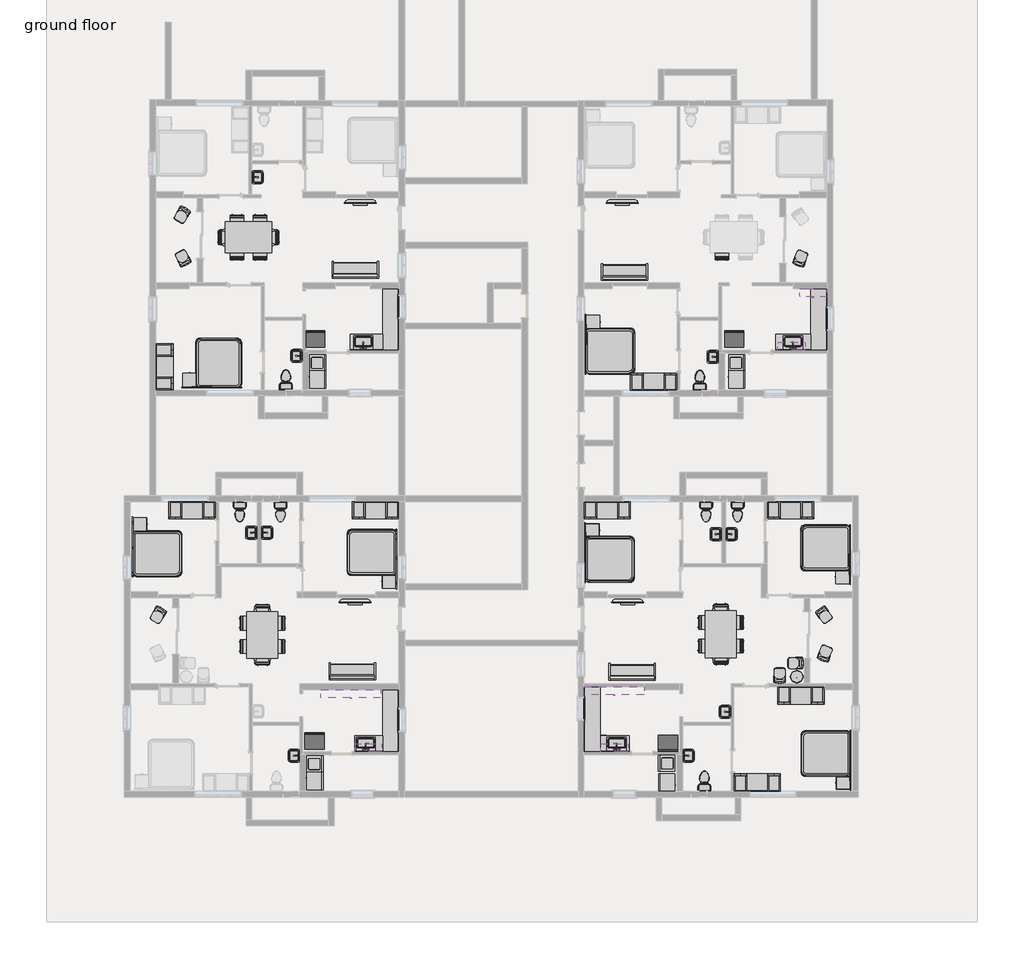
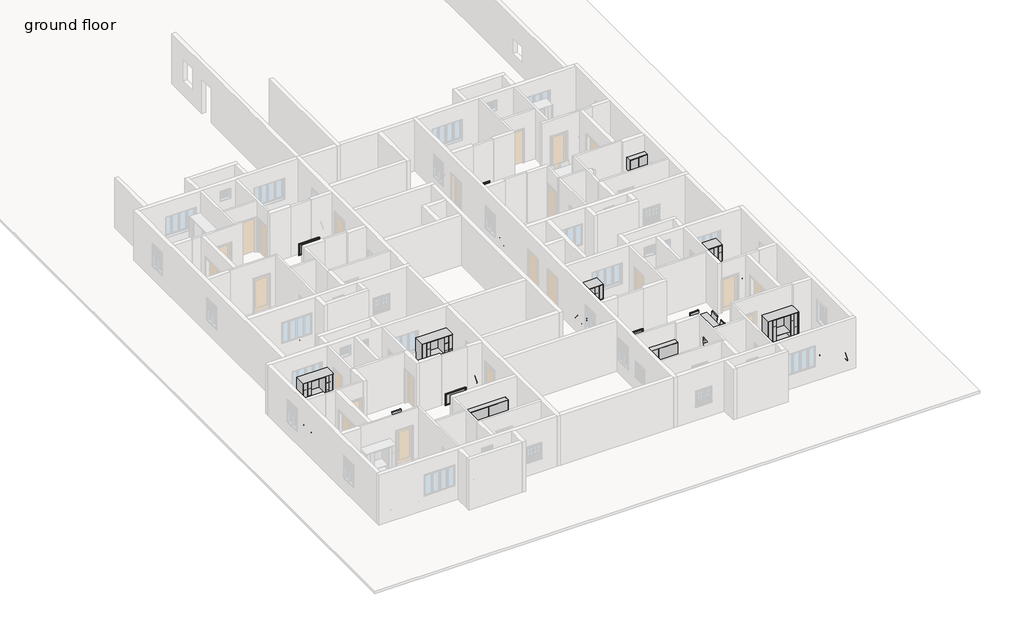
# One storey, part 11 of 16: 80 furniture elements, 21 flow terminals, 12 proxies.
"""IFC4 building model written with IfcOpenShell, lengths in millimetres."""

from ifc_helpers import new_model, si_unit, origin, place, context, project, spatial, transform, mapped, element, save
from components import proxy_97c73763, proxy_19935bb1, proxy_76352e5b, proxy_1934c8a4, flow_terminal_4d548711, flow_terminal_8d9ea526, toilet_domestic_3d_toilet_domestic_3d_ba6479b0, toilet_domestic_3d_toilet_domestic_3d_30431060, bed_design_8999_bed_design_8999_9c973422, bed_design_8999_bed_design_8999_e911dec7, furniture_f87f75a4, furniture_a56de0b1, furniture_97fe820d, furniture_007fecef, chair_task_chair_task_b7f3823b, chair_task_arms_chair_task_arms_fa5a08ef, furniture_bc399e91, furniture_0b9e3d50, furniture_ce4e80af, furniture_8ade2860, furniture_1cc325eb, furniture_015143fb, furniture_88072bd9, furniture_eb3a3c23, furniture_4fdbbe14, furniture_57f9710a, furniture_0b81fedb, furniture_0bcc43ae, furniture_3dd5e188, furniture_9929ec1f, furniture_f73e1c42, furniture_a4bc473d, furniture_3df5d44a

model = new_model("IFC4")

# Units and contexts
model_context = context("Model", 3, world=origin())
ifc_project = project(units=[si_unit("LENGTHUNIT", "METRE", prefix="MILLI")], contexts=[model_context])

# Site, building, storey
site = spatial("IfcSite", under=ifc_project)
building = spatial("IfcBuilding", under=site)
storey = spatial("IfcBuildingStorey", under=building, Name="ground floor", Elevation=609.6)

# Proxies
placement = place(None, origin())
proxy_shape = proxy_97c73763(model_context)
element("IfcBuildingElementProxy", 1, Name="Dryer : 27\" x 25\" x 35\"", ObjectType="Dryer : 27\" x 25\" x 35\"", at=placement, inside=storey, context=model_context, shape_type="MappedRepresentation", body=[
    mapped(proxy_shape, transform((48815.0055897, -8570.7128329, 609.6), x_axis=(0.0, -1.0, 0.0), y_axis=(1.0, 0.0, 0.0), z_axis=(0.0, 0.0, 1.0))),
])
element("IfcBuildingElementProxy", 2, Name="Dryer : 27\" x 25\" x 35\"", ObjectType="Dryer : 27\" x 25\" x 35\"", at=placement, inside=storey, context=model_context, shape_type="MappedRepresentation", body=[
    mapped(proxy_shape, transform((65274.2055897, -8570.7128329, 609.6), x_axis=(0.0, -1.0, 0.0), y_axis=(1.0, 0.0, 0.0), z_axis=(0.0, 0.0, 1.0))),
])
element("IfcBuildingElementProxy", 3, Name="Dryer : 27\" x 25\" x 35\"", ObjectType="Dryer : 27\" x 25\" x 35\"", at=placement, inside=storey, context=model_context, shape_type="MappedRepresentation", body=[
    mapped(proxy_shape, transform((63151.1859463, -25146.6240794, 609.6), x_axis=(0.0, 1.0, 0.0), y_axis=(-1.0, 0.0, 0.0), z_axis=(0.0, 0.0, 1.0))),
])
element("IfcBuildingElementProxy", 4, Name="Dryer : 27\" x 25\" x 35\"", ObjectType="Dryer : 27\" x 25\" x 35\"", at=placement, inside=storey, context=model_context, shape_type="MappedRepresentation", body=[
    mapped(proxy_shape, transform((48702.4341432, -24333.8240794, 609.6), x_axis=(0.0, -1.0, 0.0), y_axis=(1.0, 0.0, 0.0), z_axis=(0.0, 0.0, 1.0))),
])
proxy_2_shape = proxy_19935bb1(model_context)
element("IfcBuildingElementProxy", 5, Name="Refrigerator-Built-in : 30\" x 24\" LH", ObjectType="Refrigerator-Built-in : 30\" x 24\" LH", at=placement, inside=storey, context=model_context, shape_type="MappedRepresentation", body=[
    mapped(proxy_2_shape, transform((62887.9133315, -23204.1520196, 609.6), x_axis=(1.0, 0.0, 0.0), y_axis=(0.0, 1.0, 0.0), z_axis=(0.0, 0.0, 1.0))),
])
proxy_3_shape = proxy_76352e5b(model_context)
element("IfcBuildingElementProxy", 6, Name="Refrigerator-Built-in : 30\" x 24\" LH", ObjectType="Refrigerator-Built-in : 30\" x 24\" LH", at=placement, inside=storey, context=model_context, shape_type="MappedRepresentation", body=[
    mapped(proxy_3_shape, transform((49034.332975, -7390.2407731, 609.6), x_axis=(1.0, 0.0, 0.0), y_axis=(0.0, 1.0, 0.0), z_axis=(0.0, 0.0, 1.0))),
])
element("IfcBuildingElementProxy", 7, Name="Refrigerator-Built-in : 30\" x 24\" LH", ObjectType="Refrigerator-Built-in : 30\" x 24\" LH", at=placement, inside=storey, context=model_context, shape_type="MappedRepresentation", body=[
    mapped(proxy_3_shape, transform((65493.532975, -7390.2407731, 609.6), x_axis=(1.0, 0.0, 0.0), y_axis=(0.0, 1.0, 0.0), z_axis=(0.0, 0.0, 1.0))),
])
element("IfcBuildingElementProxy", 8, Name="Refrigerator-Built-in : 30\" x 24\" LH", ObjectType="Refrigerator-Built-in : 30\" x 24\" LH", at=placement, inside=storey, context=model_context, shape_type="MappedRepresentation", body=[
    mapped(proxy_3_shape, transform((48997.9615284, -23178.7520196, 609.6), x_axis=(1.0, 0.0, 0.0), y_axis=(0.0, 1.0, 0.0), z_axis=(0.0, 0.0, 1.0))),
])
proxy_4_shape = proxy_1934c8a4(model_context)
element("IfcBuildingElementProxy", 9, Name="Washer : 25\" x 25\" x 35\"", ObjectType="Washer : 25\" x 25\" x 35\"", at=placement, inside=storey, context=model_context, shape_type="MappedRepresentation", body=[
    mapped(proxy_4_shape, transform((48850.5170287, -7894.2828207, 609.6), x_axis=(0.0, -1.0, 0.0), y_axis=(1.0, 0.0, 0.0), z_axis=(0.0, 0.0, 1.0))),
])
element("IfcBuildingElementProxy", 10, Name="Washer : 25\" x 25\" x 35\"", ObjectType="Washer : 25\" x 25\" x 35\"", at=placement, inside=storey, context=model_context, shape_type="MappedRepresentation", body=[
    mapped(proxy_4_shape, transform((65309.7170287, -7894.2828207, 609.6), x_axis=(0.0, -1.0, 0.0), y_axis=(1.0, 0.0, 0.0), z_axis=(0.0, 0.0, 1.0))),
])
element("IfcBuildingElementProxy", 11, Name="Washer : 25\" x 25\" x 35\"", ObjectType="Washer : 25\" x 25\" x 35\"", at=placement, inside=storey, context=model_context, shape_type="MappedRepresentation", body=[
    mapped(proxy_4_shape, transform((63110.4973853, -24419.3940673, 609.6), x_axis=(0.0, 1.0, 0.0), y_axis=(-1.0, 0.0, 0.0), z_axis=(0.0, 0.0, 1.0))),
])
element("IfcBuildingElementProxy", 12, Name="Washer : 25\" x 25\" x 35\"", ObjectType="Washer : 25\" x 25\" x 35\"", at=placement, inside=storey, context=model_context, shape_type="MappedRepresentation", body=[
    mapped(proxy_4_shape, transform((48737.9455822, -23657.3940673, 609.6), x_axis=(0.0, -1.0, 0.0), y_axis=(1.0, 0.0, 0.0), z_axis=(0.0, 0.0, 1.0))),
])

# Flow terminals
flow_terminal_shape = flow_terminal_4d548711(model_context)
element("IfcFlowTerminal", 13, ObjectType="Sink Kitchen-Single : 30\" x 21\"", at=placement, inside=storey, context=model_context, shape_type="MappedRepresentation", body=[
    mapped(flow_terminal_shape, transform((50929.549914, -7494.5659653, 609.6), x_axis=(-1.0, 0.0, 0.0), y_axis=(0.0, -1.0, 0.0), z_axis=(0.0, 0.0, 1.0))),
])
element("IfcFlowTerminal", 14, ObjectType="Sink Kitchen-Single : 30\" x 21\"", at=placement, inside=storey, context=model_context, shape_type="MappedRepresentation", body=[
    mapped(flow_terminal_shape, transform((67814.4575644, -7494.5659653, 609.6), x_axis=(-1.0, 0.0, 0.0), y_axis=(0.0, -1.0, 0.0), z_axis=(0.0, 0.0, 1.0))),
])
element("IfcFlowTerminal", 15, ObjectType="Sink Kitchen-Single : 30\" x 21\"", at=placement, inside=storey, context=model_context, shape_type="MappedRepresentation", body=[
    mapped(flow_terminal_shape, transform((60886.6970546, -23264.1704575, 609.6), x_axis=(-1.0, 0.0, 0.0), y_axis=(0.0, -1.0, 0.0), z_axis=(0.0, 0.0, 1.0))),
])
element("IfcFlowTerminal", 16, ObjectType="Sink Kitchen-Single : 30\" x 21\"", at=placement, inside=storey, context=model_context, shape_type="MappedRepresentation", body=[
    mapped(flow_terminal_shape, transform((51027.9054731, -23264.2911897, 609.6), x_axis=(-1.0, 0.0, 0.0), y_axis=(0.0, -1.0, 0.0), z_axis=(0.0, 0.0, 1.0))),
])
flow_terminal_2_shape = flow_terminal_8d9ea526(model_context)
element("IfcFlowTerminal", 17, ObjectType="Sink Vanity-Square : 20\" x 18\"", at=placement, inside=storey, context=model_context, shape_type="MappedRepresentation", body=[
    mapped(flow_terminal_2_shape, transform((64700.8858807, -8040.0221259, 609.6), x_axis=(0.0, -1.0, 0.0), y_axis=(1.0, 0.0, 0.0), z_axis=(0.0, 0.0, 1.0))),
])
element("IfcFlowTerminal", 18, ObjectType="Sink Vanity-Square : 20\" x 18\"", at=placement, inside=storey, context=model_context, shape_type="MappedRepresentation", body=[
    mapped(flow_terminal_2_shape, transform((64819.063292, -15003.2055572, 609.6), x_axis=(0.0, -1.0, 0.0), y_axis=(1.0, 0.0, 0.0), z_axis=(0.0, 0.0, 1.0))),
])
element("IfcFlowTerminal", 19, ObjectType="Sink Vanity-Square : 20\" x 18\"", at=placement, inside=storey, context=model_context, shape_type="MappedRepresentation", body=[
    mapped(flow_terminal_2_shape, transform((65325.5370757, -15034.5840384, 609.6), x_axis=(0.0, 1.0, 0.0), y_axis=(-1.0, 0.0, 0.0), z_axis=(0.0, 0.0, 1.0))),
])
element("IfcFlowTerminal", 20, ObjectType="Sink Vanity-Square : 20\" x 18\"", at=placement, inside=storey, context=model_context, shape_type="MappedRepresentation", body=[
    mapped(flow_terminal_2_shape, transform((65180.5928441, -21983.9881535, 609.6), x_axis=(0.0, -1.0, 0.0), y_axis=(1.0, 0.0, 0.0), z_axis=(0.0, 0.0, 1.0))),
])
element("IfcFlowTerminal", 21, ObjectType="Sink Vanity-Square : 20\" x 18\"", at=placement, inside=storey, context=model_context, shape_type="MappedRepresentation", body=[
    mapped(flow_terminal_2_shape, transform((63638.776683, -23739.4050992, 609.6), x_axis=(0.0, 1.0, 0.0), y_axis=(-1.0, 0.0, 0.0), z_axis=(0.0, 0.0, 1.0))),
])
element("IfcFlowTerminal", 22, ObjectType="Sink Vanity-Square : 20\" x 18\"", at=placement, inside=storey, context=model_context, shape_type="MappedRepresentation", body=[
    mapped(flow_terminal_2_shape, transform((48244.6808419, -23708.1473503, 609.6), x_axis=(0.0, -1.0, 0.0), y_axis=(1.0, 0.0, 0.0), z_axis=(0.0, 0.0, 1.0))),
])
element("IfcFlowTerminal", 23, ObjectType="Sink Vanity-Square : 20\" x 18\"", at=placement, inside=storey, context=model_context, shape_type="MappedRepresentation", body=[
    mapped(flow_terminal_2_shape, transform((46567.622986, -14945.2984998, 609.6), x_axis=(0.0, -1.0, 0.0), y_axis=(1.0, 0.0, 0.0), z_axis=(0.0, 0.0, 1.0))),
])
element("IfcFlowTerminal", 24, ObjectType="Sink Vanity-Square : 20\" x 18\"", at=placement, inside=storey, context=model_context, shape_type="MappedRepresentation", body=[
    mapped(flow_terminal_2_shape, transform((47080.9674776, -14976.676981, 609.6), x_axis=(0.0, 1.0, 0.0), y_axis=(-1.0, 0.0, 0.0), z_axis=(0.0, 0.0, 1.0))),
])
element("IfcFlowTerminal", 25, ObjectType="Sink Vanity-Square : 20\" x 18\"", at=placement, inside=storey, context=model_context, shape_type="MappedRepresentation", body=[
    mapped(flow_terminal_2_shape, transform((48339.9308419, -8001.9221259, 609.6), x_axis=(0.0, -1.0, 0.0), y_axis=(1.0, 0.0, 0.0), z_axis=(0.0, 0.0, 1.0))),
])
element("IfcFlowTerminal", 26, ObjectType="Sink Vanity-Square : 20\" x 18\"", at=placement, inside=storey, context=model_context, shape_type="MappedRepresentation", body=[
    mapped(flow_terminal_2_shape, transform((46712.6716441, -1008.3845426, 609.6), x_axis=(0.0, 1.0, 0.0), y_axis=(-1.0, 0.0, 0.0), z_axis=(0.0, 0.0, 1.0))),
])
toilet_domestic_3d_toilet_domestic_3d_shape = toilet_domestic_3d_toilet_domestic_3d_ba6479b0(model_context)
toilet_domestic_3d_toilet_domestic_3d_2_shape = toilet_domestic_3d_toilet_domestic_3d_30431060(model_context)
element("IfcFlowTerminal", 27, ObjectType="Toilet-Domestic-3D : Toilet-Domestic-3D", at=placement, inside=storey, context=model_context, shape_type="MappedRepresentation", body=[
    mapped(toilet_domestic_3d_toilet_domestic_3d_shape, transform((64138.0812819, -8877.446445, 609.6), x_axis=(-1.0, 0.0, 0.0), y_axis=(0.0, -1.0, 0.0), z_axis=(0.0, 0.0, 1.0))),
    mapped(toilet_domestic_3d_toilet_domestic_3d_2_shape, transform((64138.0812819, -8877.446445, 609.6), x_axis=(-1.0, 0.0, 0.0), y_axis=(0.0, -1.0, 0.0), z_axis=(0.0, 0.0, 1.0))),
])
element("IfcFlowTerminal", 28, ObjectType="Toilet-Domestic-3D : Toilet-Domestic-3D", at=placement, inside=storey, context=model_context, shape_type="MappedRepresentation", body=[
    mapped(toilet_domestic_3d_toilet_domestic_3d_shape, transform((47872.376243, -8863.029317, 609.6), x_axis=(-1.0, 0.0, 0.0), y_axis=(0.0, -1.0, 0.0), z_axis=(0.0, 0.0, 1.0))),
    mapped(toilet_domestic_3d_toilet_domestic_3d_2_shape, transform((47872.376243, -8863.029317, 609.6), x_axis=(-1.0, 0.0, 0.0), y_axis=(0.0, -1.0, 0.0), z_axis=(0.0, 0.0, 1.0))),
])
element("IfcFlowTerminal", 29, ObjectType="Toilet-Domestic-3D : Toilet-Domestic-3D", at=placement, inside=storey, context=model_context, shape_type="MappedRepresentation", body=[
    mapped(toilet_domestic_3d_toilet_domestic_3d_shape, transform((47662.826243, -14236.3326182, 609.6), x_axis=(1.0, 0.0, 0.0), y_axis=(0.0, 1.0, 0.0), z_axis=(0.0, 0.0, 1.0))),
    mapped(toilet_domestic_3d_toilet_domestic_3d_2_shape, transform((47662.826243, -14236.3326182, 609.6), x_axis=(1.0, 0.0, 0.0), y_axis=(0.0, 1.0, 0.0), z_axis=(0.0, 0.0, 1.0))),
])
element("IfcFlowTerminal", 30, ObjectType="Toilet-Domestic-3D : Toilet-Domestic-3D", at=placement, inside=storey, context=model_context, shape_type="MappedRepresentation", body=[
    mapped(toilet_domestic_3d_toilet_domestic_3d_shape, transform((46062.626243, -14236.3326182, 609.6), x_axis=(1.0, 0.0, 0.0), y_axis=(0.0, 1.0, 0.0), z_axis=(0.0, 0.0, 1.0))),
    mapped(toilet_domestic_3d_toilet_domestic_3d_2_shape, transform((46062.626243, -14236.3326182, 609.6), x_axis=(1.0, 0.0, 0.0), y_axis=(0.0, 1.0, 0.0), z_axis=(0.0, 0.0, 1.0))),
])
element("IfcFlowTerminal", 31, ObjectType="Toilet-Domestic-3D : Toilet-Domestic-3D", at=placement, inside=storey, context=model_context, shape_type="MappedRepresentation", body=[
    mapped(toilet_domestic_3d_toilet_domestic_3d_shape, transform((64315.8812819, -24626.1405635, 609.6), x_axis=(-1.0, 0.0, 0.0), y_axis=(0.0, -1.0, 0.0), z_axis=(0.0, 0.0, 1.0))),
    mapped(toilet_domestic_3d_toilet_domestic_3d_2_shape, transform((64315.8812819, -24626.1405635, 609.6), x_axis=(-1.0, 0.0, 0.0), y_axis=(0.0, -1.0, 0.0), z_axis=(0.0, 0.0, 1.0))),
])
element("IfcFlowTerminal", 32, ObjectType="Toilet-Domestic-3D : Toilet-Domestic-3D", at=placement, inside=storey, context=model_context, shape_type="MappedRepresentation", body=[
    mapped(toilet_domestic_3d_toilet_domestic_3d_shape, transform((64385.7312819, -14236.3326182, 609.6), x_axis=(1.0, 0.0, 0.0), y_axis=(0.0, 1.0, 0.0), z_axis=(0.0, 0.0, 1.0))),
    mapped(toilet_domestic_3d_toilet_domestic_3d_2_shape, transform((64385.7312819, -14236.3326182, 609.6), x_axis=(1.0, 0.0, 0.0), y_axis=(0.0, 1.0, 0.0), z_axis=(0.0, 0.0, 1.0))),
])
element("IfcFlowTerminal", 33, ObjectType="Toilet-Domestic-3D : Toilet-Domestic-3D", at=placement, inside=storey, context=model_context, shape_type="MappedRepresentation", body=[
    mapped(toilet_domestic_3d_toilet_domestic_3d_shape, transform((65622.4515239, -14236.3326182, 609.6), x_axis=(1.0, 0.0, 0.0), y_axis=(0.0, 1.0, 0.0), z_axis=(0.0, 0.0, 1.0))),
    mapped(toilet_domestic_3d_toilet_domestic_3d_2_shape, transform((65622.4515239, -14236.3326182, 609.6), x_axis=(1.0, 0.0, 0.0), y_axis=(0.0, 1.0, 0.0), z_axis=(0.0, 0.0, 1.0))),
])

# Furniture
bed_design_8999_bed_design_8999_shape = bed_design_8999_bed_design_8999_9c973422(model_context)
bed_design_8999_bed_design_8999_2_shape = bed_design_8999_bed_design_8999_e911dec7(model_context)
element("IfcFurniture", 34, ObjectType="BED_DESIGN_8999 : BED_DESIGN_8999", at=placement, inside=storey, context=model_context, shape_type="MappedRepresentation", body=[
    mapped(bed_design_8999_bed_design_8999_shape, transform((61579.0312819, -7630.2613664, 609.6), x_axis=(0.0, 1.0, 0.0), y_axis=(-1.0, 0.0, 0.0), z_axis=(0.0, 0.0, 1.0))),
    mapped(bed_design_8999_bed_design_8999_2_shape, transform((61579.0312819, -7630.2613664, 609.6), x_axis=(0.0, 1.0, 0.0), y_axis=(-1.0, 0.0, 0.0), z_axis=(0.0, 0.0, 1.0))),
])
element("IfcFurniture", 35, ObjectType="BED_DESIGN_8999 : BED_DESIGN_8999", at=placement, inside=storey, context=model_context, shape_type="MappedRepresentation", body=[
    mapped(bed_design_8999_bed_design_8999_shape, transform((61566.3320439, -15811.7365909, 609.6), x_axis=(0.0, 1.0, 0.0), y_axis=(-1.0, 0.0, 0.0), z_axis=(0.0, 0.0, 1.0))),
    mapped(bed_design_8999_bed_design_8999_2_shape, transform((61566.3320439, -15811.7365909, 609.6), x_axis=(0.0, 1.0, 0.0), y_axis=(-1.0, 0.0, 0.0), z_axis=(0.0, 0.0, 1.0))),
])
element("IfcFurniture", 36, ObjectType="BED_DESIGN_8999 : BED_DESIGN_8999", at=placement, inside=storey, context=model_context, shape_type="MappedRepresentation", body=[
    mapped(bed_design_8999_bed_design_8999_shape, transform((68106.8305199, -15754.5865909, 609.6), x_axis=(0.0, -1.0, 0.0), y_axis=(1.0, 0.0, 0.0), z_axis=(0.0, 0.0, 1.0))),
    mapped(bed_design_8999_bed_design_8999_2_shape, transform((68106.8305199, -15754.5865909, 609.6), x_axis=(0.0, -1.0, 0.0), y_axis=(1.0, 0.0, 0.0), z_axis=(0.0, 0.0, 1.0))),
])
element("IfcFurniture", 37, ObjectType="BED_DESIGN_8999 : BED_DESIGN_8999", at=placement, inside=storey, context=model_context, shape_type="MappedRepresentation", body=[
    mapped(bed_design_8999_bed_design_8999_shape, transform((68119.5312819, -23838.1365909, 609.6), x_axis=(0.0, -1.0, 0.0), y_axis=(1.0, 0.0, 0.0), z_axis=(0.0, 0.0, 1.0))),
    mapped(bed_design_8999_bed_design_8999_2_shape, transform((68119.5312819, -23838.1365909, 609.6), x_axis=(0.0, -1.0, 0.0), y_axis=(1.0, 0.0, 0.0), z_axis=(0.0, 0.0, 1.0))),
])
element("IfcFurniture", 38, ObjectType="BED_DESIGN_8999 : BED_DESIGN_8999", at=placement, inside=storey, context=model_context, shape_type="MappedRepresentation", body=[
    mapped(bed_design_8999_bed_design_8999_shape, transform((43789.327005, -15583.1365909, 609.6), x_axis=(0.0, 1.0, 0.0), y_axis=(-1.0, 0.0, 0.0), z_axis=(0.0, 0.0, 1.0))),
    mapped(bed_design_8999_bed_design_8999_2_shape, transform((43789.327005, -15583.1365909, 609.6), x_axis=(0.0, 1.0, 0.0), y_axis=(-1.0, 0.0, 0.0), z_axis=(0.0, 0.0, 1.0))),
])
element("IfcFurniture", 39, ObjectType="BED_DESIGN_8999 : BED_DESIGN_8999", at=placement, inside=storey, context=model_context, shape_type="MappedRepresentation", body=[
    mapped(bed_design_8999_bed_design_8999_shape, transform((50279.025481, -15932.3865909, 609.6), x_axis=(0.0, -1.0, 0.0), y_axis=(1.0, 0.0, 0.0), z_axis=(0.0, 0.0, 1.0))),
    mapped(bed_design_8999_bed_design_8999_2_shape, transform((50279.025481, -15932.3865909, 609.6), x_axis=(0.0, -1.0, 0.0), y_axis=(1.0, 0.0, 0.0), z_axis=(0.0, 0.0, 1.0))),
])
element("IfcFurniture", 40, ObjectType="BED_DESIGN_8999 : BED_DESIGN_8999", at=placement, inside=storey, context=model_context, shape_type="MappedRepresentation", body=[
    mapped(bed_design_8999_bed_design_8999_shape, transform((45033.926243, -7325.4613664, 609.6), x_axis=(-1.0, 0.0, 0.0), y_axis=(0.0, -1.0, 0.0), z_axis=(0.0, 0.0, 1.0))),
    mapped(bed_design_8999_bed_design_8999_2_shape, transform((45033.926243, -7325.4613664, 609.6), x_axis=(-1.0, 0.0, 0.0), y_axis=(0.0, -1.0, 0.0), z_axis=(0.0, 0.0, 1.0))),
])
furniture_shape = furniture_f87f75a4(model_context)
element("IfcFurniture", 41, ObjectType="Base Cabinet-Combo01 : 30\"", at=placement, inside=storey, context=model_context, shape_type="MappedRepresentation", body=[
    mapped(furniture_shape, transform((69135.5312819, -5725.1603342, 609.6), x_axis=(0.0, -1.0, 0.0), y_axis=(1.0, 0.0, 0.0), z_axis=(0.0, 0.0, 1.0))),
])
element("IfcFurniture", 42, ObjectType="Base Cabinet-Combo01 : 30\"", at=placement, inside=storey, context=model_context, shape_type="MappedRepresentation", body=[
    mapped(furniture_shape, transform((69135.5312819, -6487.1603342, 609.6), x_axis=(0.0, -1.0, 0.0), y_axis=(1.0, 0.0, 0.0), z_axis=(0.0, 0.0, 1.0))),
])
element("IfcFurniture", 43, ObjectType="Base Cabinet-Combo01 : 30\"", at=placement, inside=storey, context=model_context, shape_type="MappedRepresentation", body=[
    mapped(furniture_shape, transform((52311.026243, -5725.1603342, 609.6), x_axis=(0.0, -1.0, 0.0), y_axis=(1.0, 0.0, 0.0), z_axis=(0.0, 0.0, 1.0))),
])
element("IfcFurniture", 44, ObjectType="Base Cabinet-Combo01 : 30\"", at=placement, inside=storey, context=model_context, shape_type="MappedRepresentation", body=[
    mapped(furniture_shape, transform((52311.026243, -6487.1603342, 609.6), x_axis=(0.0, -1.0, 0.0), y_axis=(1.0, 0.0, 0.0), z_axis=(0.0, 0.0, 1.0))),
])
element("IfcFurniture", 45, ObjectType="Base Cabinet-Combo01 : 30\"", at=placement, inside=storey, context=model_context, shape_type="MappedRepresentation", body=[
    mapped(furniture_shape, transform((52311.026243, -21494.8855586, 609.6), x_axis=(0.0, -1.0, 0.0), y_axis=(1.0, 0.0, 0.0), z_axis=(0.0, 0.0, 1.0))),
])
element("IfcFurniture", 46, ObjectType="Base Cabinet-Combo01 : 30\"", at=placement, inside=storey, context=model_context, shape_type="MappedRepresentation", body=[
    mapped(furniture_shape, transform((52311.026243, -22256.8855586, 609.6), x_axis=(0.0, -1.0, 0.0), y_axis=(1.0, 0.0, 0.0), z_axis=(0.0, 0.0, 1.0))),
])
furniture_2_shape = furniture_a56de0b1(model_context)
element("IfcFurniture", 47, ObjectType="Base Cabinet-Combo01 : 30\"", at=placement, inside=storey, context=model_context, shape_type="MappedRepresentation", body=[
    mapped(furniture_2_shape, transform((59575.426243, -21469.4855586, 609.6), x_axis=(0.0, -1.0, 0.0), y_axis=(1.0, 0.0, 0.0), z_axis=(0.0, 0.0, 1.0))),
])
element("IfcFurniture", 48, ObjectType="Base Cabinet-Combo01 : 30\"", at=placement, inside=storey, context=model_context, shape_type="MappedRepresentation", body=[
    mapped(furniture_2_shape, transform((59575.426243, -22231.4855586, 609.6), x_axis=(0.0, -1.0, 0.0), y_axis=(1.0, 0.0, 0.0), z_axis=(0.0, 0.0, 1.0))),
])
furniture_3_shape = furniture_97fe820d(model_context)
element("IfcFurniture", 49, ObjectType="Base Cabinet-Corner Unit-Square : 36\"", at=placement, inside=storey, context=model_context, shape_type="MappedRepresentation", body=[
    mapped(furniture_3_shape, transform((69135.5312819, -7275.1849244, 609.6), x_axis=(0.0, -1.0, 0.0), y_axis=(1.0, 0.0, 0.0), z_axis=(0.0, 0.0, 1.0))),
])
element("IfcFurniture", 50, ObjectType="Base Cabinet-Corner Unit-Square : 36\"", at=placement, inside=storey, context=model_context, shape_type="MappedRepresentation", body=[
    mapped(furniture_3_shape, transform((52311.026243, -7275.1849244, 609.6), x_axis=(0.0, -1.0, 0.0), y_axis=(1.0, 0.0, 0.0), z_axis=(0.0, 0.0, 1.0))),
])
element("IfcFurniture", 51, ObjectType="Base Cabinet-Corner Unit-Square : 36\"", at=placement, inside=storey, context=model_context, shape_type="MappedRepresentation", body=[
    mapped(furniture_3_shape, transform((52311.026243, -23044.9101488, 609.6), x_axis=(0.0, -1.0, 0.0), y_axis=(1.0, 0.0, 0.0), z_axis=(0.0, 0.0, 1.0))),
])
furniture_4_shape = furniture_007fecef(model_context)
element("IfcFurniture", 52, ObjectType="Base Cabinet-Corner Unit-Square : 36\"", at=placement, inside=storey, context=model_context, shape_type="MappedRepresentation", body=[
    mapped(furniture_4_shape, transform((59575.426243, -23019.5101488, 609.6), x_axis=(0.0, -1.0, 0.0), y_axis=(1.0, 0.0, 0.0), z_axis=(0.0, 0.0, 1.0))),
])
chair_task_chair_task_shape = chair_task_chair_task_b7f3823b(model_context)
element("IfcFurniture", 53, ObjectType="Chair-Task : Chair-Task", at=placement, inside=storey, context=model_context, shape_type="MappedRepresentation", body=[
    mapped(chair_task_chair_task_shape, transform((64873.3904622, -3989.5848828, 609.6), x_axis=(1.0, 0.0, 0.0), y_axis=(0.0, 1.0, 0.0), z_axis=(0.0, 0.0, 1.0))),
])
element("IfcFurniture", 54, ObjectType="Chair-Task : Chair-Task", at=placement, inside=storey, context=model_context, shape_type="MappedRepresentation", body=[
    mapped(chair_task_chair_task_shape, transform((45807.3354234, -3989.5848828, 609.6), x_axis=(1.0, 0.0, 0.0), y_axis=(0.0, 1.0, 0.0), z_axis=(0.0, 0.0, 1.0))),
])
element("IfcFurniture", 55, ObjectType="Chair-Task : Chair-Task", at=placement, inside=storey, context=model_context, shape_type="MappedRepresentation", body=[
    mapped(chair_task_chair_task_shape, transform((46089.3170627, -2732.4930795, 609.6), x_axis=(-1.0, 0.0, 0.0), y_axis=(0.0, -1.0, 0.0), z_axis=(0.0, 0.0, 1.0))),
])
element("IfcFurniture", 56, ObjectType="Chair-Task : Chair-Task", at=placement, inside=storey, context=model_context, shape_type="MappedRepresentation", body=[
    mapped(chair_task_chair_task_shape, transform((46721.7354234, -3989.5848828, 609.6), x_axis=(1.0, 0.0, 0.0), y_axis=(0.0, 1.0, 0.0), z_axis=(0.0, 0.0, 1.0))),
])
element("IfcFurniture", 57, ObjectType="Chair-Task : Chair-Task", at=placement, inside=storey, context=model_context, shape_type="MappedRepresentation", body=[
    mapped(chair_task_chair_task_shape, transform((47003.7170627, -2732.4930795, 609.6), x_axis=(-1.0, 0.0, 0.0), y_axis=(0.0, -1.0, 0.0), z_axis=(0.0, 0.0, 1.0))),
])
element("IfcFurniture", 58, ObjectType="Chair-Task : Chair-Task", at=placement, inside=storey, context=model_context, shape_type="MappedRepresentation", body=[
    mapped(chair_task_chair_task_shape, transform((47580.1721447, -19574.3567408, 609.6), x_axis=(0.0, 1.0, 0.0), y_axis=(-1.0, 0.0, 0.0), z_axis=(0.0, 0.0, 1.0))),
])
element("IfcFurniture", 59, ObjectType="Chair-Task : Chair-Task", at=placement, inside=storey, context=model_context, shape_type="MappedRepresentation", body=[
    mapped(chair_task_chair_task_shape, transform((46323.0803414, -19292.3751014, 609.6), x_axis=(0.0, -1.0, 0.0), y_axis=(1.0, 0.0, 0.0), z_axis=(0.0, 0.0, 1.0))),
])
element("IfcFurniture", 60, ObjectType="Chair-Task : Chair-Task", at=placement, inside=storey, context=model_context, shape_type="MappedRepresentation", body=[
    mapped(chair_task_chair_task_shape, transform((47580.1721447, -18659.9567408, 609.6), x_axis=(0.0, 1.0, 0.0), y_axis=(-1.0, 0.0, 0.0), z_axis=(0.0, 0.0, 1.0))),
])
element("IfcFurniture", 61, ObjectType="Chair-Task : Chair-Task", at=placement, inside=storey, context=model_context, shape_type="MappedRepresentation", body=[
    mapped(chair_task_chair_task_shape, transform((46323.0803414, -18377.9751014, 609.6), x_axis=(0.0, -1.0, 0.0), y_axis=(1.0, 0.0, 0.0), z_axis=(0.0, 0.0, 1.0))),
])
element("IfcFurniture", 62, ObjectType="Chair-Task : Chair-Task", at=placement, inside=storey, context=model_context, shape_type="MappedRepresentation", body=[
    mapped(chair_task_chair_task_shape, transform((65592.7875464, -19549.8247856, 609.6), x_axis=(0.0, 1.0, 0.0), y_axis=(-1.0, 0.0, 0.0), z_axis=(0.0, 0.0, 1.0))),
])
element("IfcFurniture", 63, ObjectType="Chair-Task : Chair-Task", at=placement, inside=storey, context=model_context, shape_type="MappedRepresentation", body=[
    mapped(chair_task_chair_task_shape, transform((64335.6957432, -19267.8431462, 609.6), x_axis=(0.0, -1.0, 0.0), y_axis=(1.0, 0.0, 0.0), z_axis=(0.0, 0.0, 1.0))),
])
element("IfcFurniture", 64, ObjectType="Chair-Task : Chair-Task", at=placement, inside=storey, context=model_context, shape_type="MappedRepresentation", body=[
    mapped(chair_task_chair_task_shape, transform((65592.7875464, -18635.4247856, 609.6), x_axis=(0.0, 1.0, 0.0), y_axis=(-1.0, 0.0, 0.0), z_axis=(0.0, 0.0, 1.0))),
])
element("IfcFurniture", 65, ObjectType="Chair-Task : Chair-Task", at=placement, inside=storey, context=model_context, shape_type="MappedRepresentation", body=[
    mapped(chair_task_chair_task_shape, transform((64335.6957432, -18353.4431462, 609.6), x_axis=(0.0, -1.0, 0.0), y_axis=(1.0, 0.0, 0.0), z_axis=(0.0, 0.0, 1.0))),
])
chair_task_arms_chair_task_arms_shape = chair_task_arms_chair_task_arms_fa5a08ef(model_context)
element("IfcFurniture", 66, ObjectType="Chair-Task Arms : Chair-Task Arms", at=placement, inside=storey, context=model_context, shape_type="MappedRepresentation", body=[
    mapped(chair_task_arms_chair_task_arms_shape, transform((47338.8721447, -3502.0298008, 609.6), x_axis=(0.0, 1.0, 0.0), y_axis=(-1.0, 0.0, 0.0), z_axis=(0.0, 0.0, 1.0))),
])
element("IfcFurniture", 67, ObjectType="Chair-Task Arms : Chair-Task Arms", at=placement, inside=storey, context=model_context, shape_type="MappedRepresentation", body=[
    mapped(chair_task_arms_chair_task_arms_shape, transform((45472.1803414, -3220.0481615, 609.6), x_axis=(0.0, -1.0, 0.0), y_axis=(1.0, 0.0, 0.0), z_axis=(0.0, 0.0, 1.0))),
])
element("IfcFurniture", 68, ObjectType="Chair-Task Arms : Chair-Task Arms", at=placement, inside=storey, context=model_context, shape_type="MappedRepresentation", body=[
    mapped(chair_task_arms_chair_task_arms_shape, transform((47092.6170627, -18042.8200195, 609.6), x_axis=(-1.0, 0.0, 0.0), y_axis=(0.0, -1.0, 0.0), z_axis=(0.0, 0.0, 1.0))),
])
element("IfcFurniture", 69, ObjectType="Chair-Task Arms : Chair-Task Arms", at=placement, inside=storey, context=model_context, shape_type="MappedRepresentation", body=[
    mapped(chair_task_arms_chair_task_arms_shape, transform((46810.6354234, -19909.5118227, 609.6), x_axis=(1.0, 0.0, 0.0), y_axis=(0.0, 1.0, 0.0), z_axis=(0.0, 0.0, 1.0))),
])
element("IfcFurniture", 70, ObjectType="Chair-Task Arms : Chair-Task Arms", at=placement, inside=storey, context=model_context, shape_type="MappedRepresentation", body=[
    mapped(chair_task_arms_chair_task_arms_shape, transform((65105.2324645, -18018.2880643, 609.6), x_axis=(-1.0, 0.0, 0.0), y_axis=(0.0, -1.0, 0.0), z_axis=(0.0, 0.0, 1.0))),
])
element("IfcFurniture", 71, ObjectType="Chair-Task Arms : Chair-Task Arms", at=placement, inside=storey, context=model_context, shape_type="MappedRepresentation", body=[
    mapped(chair_task_arms_chair_task_arms_shape, transform((64823.2508251, -19884.9798675, 609.6), x_axis=(1.0, 0.0, 0.0), y_axis=(0.0, 1.0, 0.0), z_axis=(0.0, 0.0, 1.0))),
])
furniture_5_shape = furniture_bc399e91(model_context)
element("IfcFurniture", 72, ObjectType="Counter Top : 24\" Depth", at=placement, inside=storey, context=model_context, shape_type="MappedRepresentation", body=[
    mapped(furniture_5_shape, transform((69135.5312819, -6576.4736615, 609.6), x_axis=(0.0, -1.0, 0.0), y_axis=(1.0, 0.0, 0.0), z_axis=(0.0, 0.0, 1.0))),
])
element("IfcFurniture", 73, ObjectType="Counter Top : 24\" Depth", at=placement, inside=storey, context=model_context, shape_type="MappedRepresentation", body=[
    mapped(furniture_5_shape, transform((52311.026243, -6576.4736615, 609.6), x_axis=(0.0, -1.0, 0.0), y_axis=(1.0, 0.0, 0.0), z_axis=(0.0, 0.0, 1.0))),
])
element("IfcFurniture", 74, ObjectType="Counter Top : 24\" Depth", at=placement, inside=storey, context=model_context, shape_type="MappedRepresentation", body=[
    mapped(furniture_5_shape, transform((52311.026243, -22333.4988859, 609.6), x_axis=(0.0, -1.0, 0.0), y_axis=(1.0, 0.0, 0.0), z_axis=(0.0, 0.0, 1.0))),
])
furniture_6_shape = furniture_0b9e3d50(model_context)
element("IfcFurniture", 75, ObjectType="Counter Top : 24\" Depth", at=placement, inside=storey, context=model_context, shape_type="MappedRepresentation", body=[
    mapped(furniture_6_shape, transform((59585.1312819, -22370.8535635, 609.6), x_axis=(0.0, 1.0, 0.0), y_axis=(-1.0, 0.0, 0.0), z_axis=(0.0, 0.0, 1.0))),
])
furniture_7_shape = furniture_ce4e80af(model_context)
element("IfcFurniture", 76, ObjectType="Counter Top w Sink Hole : 24\" Depth", at=placement, inside=storey, context=model_context, shape_type="MappedRepresentation", body=[
    mapped(furniture_7_shape, transform((60165.7138781, -23571.3158586, 609.6), x_axis=(-1.0, 0.0, 0.0), y_axis=(0.0, -1.0, 0.0), z_axis=(0.0, 0.0, 1.0))),
])
furniture_8_shape = furniture_8ade2860(model_context)
element("IfcFurniture", 77, ObjectType="Counter Top w Sink Hole : 24\" Depth", at=placement, inside=storey, context=model_context, shape_type="MappedRepresentation", body=[
    mapped(furniture_8_shape, transform((50475.5639479, -23571.4365909, 609.6), x_axis=(-1.0, 0.0, 0.0), y_axis=(0.0, -1.0, 0.0), z_axis=(0.0, 0.0, 1.0))),
])
furniture_9_shape = furniture_1cc325eb(model_context)
element("IfcFurniture", 78, ObjectType="Counter Top w Sink Hole : 24\" Depth", at=placement, inside=storey, context=model_context, shape_type="MappedRepresentation", body=[
    mapped(furniture_9_shape, transform((50475.5639479, -7801.7113664, 609.6), x_axis=(-1.0, 0.0, 0.0), y_axis=(0.0, -1.0, 0.0), z_axis=(0.0, 0.0, 1.0))),
])
furniture_10_shape = furniture_015143fb(model_context)
element("IfcFurniture", 79, ObjectType="Counter Top w Sink Hole : 24\" Depth", at=placement, inside=storey, context=model_context, shape_type="MappedRepresentation", body=[
    mapped(furniture_10_shape, transform((67300.0689868, -7801.7113664, 609.6), x_axis=(-1.0, 0.0, 0.0), y_axis=(0.0, -1.0, 0.0), z_axis=(0.0, 0.0, 1.0))),
])
furniture_11_shape = furniture_88072bd9(model_context)
element("IfcFurniture", 80, ObjectType="Entertainment Center : 72\" x 72\" x 24\"", at=placement, inside=storey, context=model_context, shape_type="MappedRepresentation", body=[
    mapped(furniture_11_shape, transform((62328.3312819, -9473.7424723, 609.6), x_axis=(-1.0, 0.0, 0.0), y_axis=(0.0, -1.0, 0.0), z_axis=(0.0, 0.0, 1.0))),
])
element("IfcFurniture", 81, ObjectType="Entertainment Center : 72\" x 72\" x 24\"", at=placement, inside=storey, context=model_context, shape_type="MappedRepresentation", body=[
    mapped(furniture_11_shape, transform((67700.4312819, -13640.0365909, 609.6), x_axis=(1.0, 0.0, 0.0), y_axis=(0.0, 1.0, 0.0), z_axis=(0.0, 0.0, 1.0))),
])
element("IfcFurniture", 82, ObjectType="Entertainment Center : 72\" x 72\" x 24\"", at=placement, inside=storey, context=model_context, shape_type="MappedRepresentation", body=[
    mapped(furniture_11_shape, transform((60499.5312819, -13638.5365909, 609.6), x_axis=(1.0, 0.0, 0.0), y_axis=(0.0, 1.0, 0.0), z_axis=(0.0, 0.0, 1.0))),
])
element("IfcFurniture", 83, ObjectType="Entertainment Center : 72\" x 72\" x 24\"", at=placement, inside=storey, context=model_context, shape_type="MappedRepresentation", body=[
    mapped(furniture_11_shape, transform((66392.3312819, -25222.4365909, 609.6), x_axis=(-1.0, 0.0, 0.0), y_axis=(0.0, -1.0, 0.0), z_axis=(0.0, 0.0, 1.0))),
])
element("IfcFurniture", 84, ObjectType="Entertainment Center : 72\" x 72\" x 24\"", at=placement, inside=storey, context=model_context, shape_type="MappedRepresentation", body=[
    mapped(furniture_11_shape, transform((68106.8312819, -20917.0158586, 609.6), x_axis=(1.0, 0.0, 0.0), y_axis=(0.0, 1.0, 0.0), z_axis=(0.0, 0.0, 1.0))),
])
element("IfcFurniture", 85, ObjectType="Entertainment Center : 72\" x 72\" x 24\"", at=placement, inside=storey, context=model_context, shape_type="MappedRepresentation", body=[
    mapped(furniture_11_shape, transform((44195.726243, -13640.0365909, 609.6), x_axis=(1.0, 0.0, 0.0), y_axis=(0.0, 1.0, 0.0), z_axis=(0.0, 0.0, 1.0))),
])
element("IfcFurniture", 86, ObjectType="Entertainment Center : 72\" x 72\" x 24\"", at=placement, inside=storey, context=model_context, shape_type="MappedRepresentation", body=[
    mapped(furniture_11_shape, transform((51396.626243, -13640.0365909, 609.6), x_axis=(1.0, 0.0, 0.0), y_axis=(0.0, 1.0, 0.0), z_axis=(0.0, 0.0, 1.0))),
])
element("IfcFurniture", 87, ObjectType="Entertainment Center : 72\" x 72\" x 24\"", at=placement, inside=storey, context=model_context, shape_type="MappedRepresentation", body=[
    mapped(furniture_11_shape, transform((42659.026243, -8443.3253443, 609.6), x_axis=(0.0, 1.0, 0.0), y_axis=(-1.0, 0.0, 0.0), z_axis=(0.0, 0.0, 1.0))),
])
furniture_12_shape = furniture_eb3a3c23(model_context)
element("IfcFurniture", 88, ObjectType="Seating-Auditorium : 18\" x 24\" x 30\"", at=placement, inside=storey, context=model_context, shape_type="MappedRepresentation", body=[
    mapped(furniture_12_shape, transform((44035.1924565, -2377.2923727, 609.6), x_axis=(-0.8660254037844514, 0.499999999999978, 0.0), y_axis=(-0.499999999999978, -0.8660254037844514, 0.0), z_axis=(0.0, 0.0, 1.0))),
])
element("IfcFurniture", 89, ObjectType="Seating-Auditorium : 18\" x 24\" x 30\"", at=placement, inside=storey, context=model_context, shape_type="MappedRepresentation", body=[
    mapped(furniture_12_shape, transform((43776.6115363, -4430.1215598, 609.6), x_axis=(0.8974056171641766, 0.4412064803265965, 0.0), y_axis=(-0.4412064803265965, 0.8974056171641766, 0.0), z_axis=(0.0, 0.0, 1.0))),
])
element("IfcFurniture", 90, ObjectType="Seating-Auditorium : 18\" x 24\" x 30\"", at=placement, inside=storey, context=model_context, shape_type="MappedRepresentation", body=[
    mapped(furniture_12_shape, transform((43093.6599058, -18097.0299339, 609.6), x_axis=(-0.8660254037844514, 0.499999999999978, 0.0), y_axis=(-0.499999999999978, -0.8660254037844514, 0.0), z_axis=(0.0, 0.0, 1.0))),
])
furniture_13_shape = furniture_4fdbbe14(model_context)
element("IfcFurniture", 91, ObjectType="Seating-Auditorium : 18\" x 24\" x 30\"", at=placement, inside=storey, context=model_context, shape_type="MappedRepresentation", body=[
    mapped(furniture_13_shape, transform((68098.9852443, -19923.2088345, 609.6), x_axis=(0.0, -1.0, 0.0), y_axis=(1.0, 0.0, 0.0), z_axis=(0.0, 0.0, 1.0))),
])
element("IfcFurniture", 92, ObjectType="Seating-Auditorium : 18\" x 24\" x 30\"", at=placement, inside=storey, context=model_context, shape_type="MappedRepresentation", body=[
    mapped(furniture_13_shape, transform((67434.8377033, -20772.8323698, 609.6), x_axis=(-1.0, 0.0, 0.0), y_axis=(0.0, -1.0, 0.0), z_axis=(0.0, 0.0, 1.0))),
])
element("IfcFurniture", 93, ObjectType="Seating-Auditorium : 18\" x 24\" x 30\"", at=placement, inside=storey, context=model_context, shape_type="MappedRepresentation", body=[
    mapped(furniture_13_shape, transform((68778.1156319, -18124.9352954, 609.6), x_axis=(0.8090169943749633, 0.5877852522924515, 0.0), y_axis=(-0.5877852522924515, 0.8090169943749633, 0.0), z_axis=(0.0, 0.0, 1.0))),
])
element("IfcFurniture", 94, ObjectType="Seating-Auditorium : 18\" x 24\" x 30\"", at=placement, inside=storey, context=model_context, shape_type="MappedRepresentation", body=[
    mapped(furniture_13_shape, transform((69137.0824317, -19951.6262868, 609.6), x_axis=(-0.9386081706685208, 0.3449850749732413, 0.0), y_axis=(-0.3449850749732413, -0.9386081706685208, 0.0), z_axis=(0.0, 0.0, 1.0))),
])
element("IfcFurniture", 95, ObjectType="Seating-Auditorium : 18\" x 24\" x 30\"", at=placement, inside=storey, context=model_context, shape_type="MappedRepresentation", body=[
    mapped(furniture_13_shape, transform((68173.2712739, -4433.6619337, 609.6), x_axis=(-0.9386081706685208, 0.3449850749732413, 0.0), y_axis=(-0.3449850749732413, -0.9386081706685208, 0.0), z_axis=(0.0, 0.0, 1.0))),
])
furniture_14_shape = furniture_57f9710a(model_context)
element("IfcFurniture", 96, ObjectType="Sofa : 72\"", at=placement, inside=storey, context=model_context, shape_type="MappedRepresentation", body=[
    mapped(furniture_14_shape, transform((61249.8419252, -4575.8072681, 609.6), x_axis=(-1.0, 0.0, 0.0), y_axis=(0.0, -1.0, 0.0), z_axis=(0.0, 0.0, 1.0))),
])
element("IfcFurniture", 97, ObjectType="Sofa : 72\"", at=placement, inside=storey, context=model_context, shape_type="MappedRepresentation", body=[
    mapped(furniture_14_shape, transform((61547.8017737, -20281.9117603, 609.6), x_axis=(-1.0, 0.0, 0.0), y_axis=(0.0, -1.0, 0.0), z_axis=(0.0, 0.0, 1.0))),
])
element("IfcFurniture", 98, ObjectType="Sofa : 72\"", at=placement, inside=storey, context=model_context, shape_type="MappedRepresentation", body=[
    mapped(furniture_14_shape, transform((50558.9467348, -20256.6324925, 609.6), x_axis=(-1.0, 0.0, 0.0), y_axis=(0.0, -1.0, 0.0), z_axis=(0.0, 0.0, 1.0))),
])
element("IfcFurniture", 99, ObjectType="Sofa : 72\"", at=placement, inside=storey, context=model_context, shape_type="MappedRepresentation", body=[
    mapped(furniture_14_shape, transform((50674.491973, -4484.8049088, 609.6), x_axis=(-1.0, 0.0, 0.0), y_axis=(0.0, -1.0, 0.0), z_axis=(0.0, 0.0, 1.0))),
])
furniture_15_shape = furniture_0b81fedb(model_context)
element("IfcFurniture", 100, ObjectType="TV - Flat Screen : 50\"", at=placement, inside=storey, context=model_context, shape_type="MappedRepresentation", body=[
    mapped(furniture_15_shape, transform((50803.0475952, -1944.8281223, 609.6), x_axis=(1.0, 0.0, 0.0), y_axis=(0.0, 1.0, 0.0), z_axis=(0.0, 0.0, 1.0))),
])
element("IfcFurniture", 101, ObjectType="TV - Flat Screen : 50\"", at=placement, inside=storey, context=model_context, shape_type="MappedRepresentation", body=[
    mapped(furniture_15_shape, transform((61094.025796, -1944.8281223, 609.6), x_axis=(1.0, 0.0, 0.0), y_axis=(0.0, 1.0, 0.0), z_axis=(0.0, 0.0, 1.0))),
])
element("IfcFurniture", 102, ObjectType="TV - Flat Screen : 50\"", at=placement, inside=storey, context=model_context, shape_type="MappedRepresentation", body=[
    mapped(furniture_15_shape, transform((61305.5155173, -17637.9339306, 609.6), x_axis=(1.0, 0.0, 0.0), y_axis=(0.0, 1.0, 0.0), z_axis=(0.0, 0.0, 1.0))),
])
element("IfcFurniture", 103, ObjectType="TV - Flat Screen : 50\"", at=placement, inside=storey, context=model_context, shape_type="MappedRepresentation", body=[
    mapped(furniture_15_shape, transform((50598.5310359, -17637.9339306, 609.6), x_axis=(1.0, 0.0, 0.0), y_axis=(0.0, 1.0, 0.0), z_axis=(0.0, 0.0, 1.0))),
])
furniture_16_shape = furniture_0bcc43ae(model_context)
element("IfcFurniture", 104, ObjectType="Table-Conference2 w Chairs : 48\" x 144\"", at=placement, inside=storey, context=model_context, shape_type="MappedRepresentation", body=[
    mapped(furniture_16_shape, transform((46405.526243, -3361.0389812, 609.6), x_axis=(-1.0, 0.0, 0.0), y_axis=(0.0, -1.0, 0.0), z_axis=(0.0, 0.0, 1.0))),
])
element("IfcFurniture", 105, ObjectType="Table-Conference2 w Chairs : 48\" x 144\"", at=placement, inside=storey, context=model_context, shape_type="MappedRepresentation", body=[
    mapped(furniture_16_shape, transform((46951.626243, -18976.1659211, 609.6), x_axis=(0.0, -1.0, 0.0), y_axis=(1.0, 0.0, 0.0), z_axis=(0.0, 0.0, 1.0))),
])
element("IfcFurniture", 106, ObjectType="Table-Conference2 w Chairs : 48\" x 144\"", at=placement, inside=storey, context=model_context, shape_type="MappedRepresentation", body=[
    mapped(furniture_16_shape, transform((64964.2416448, -18951.6339659, 609.6), x_axis=(0.0, -1.0, 0.0), y_axis=(1.0, 0.0, 0.0), z_axis=(0.0, 0.0, 1.0))),
])
furniture_17_shape = furniture_3dd5e188(model_context)
element("IfcFurniture", 107, ObjectType="Table-Trio End : 20\" Diameter", at=placement, inside=storey, context=model_context, shape_type="MappedRepresentation", body=[
    mapped(furniture_17_shape, transform((67945.0000179, -20618.2562257, 609.6), x_axis=(-1.0, 0.0, 0.0), y_axis=(0.0, -1.0, 0.0), z_axis=(0.0, 0.0, 1.0))),
])
furniture_18_shape = furniture_9929ec1f(model_context)
element("IfcFurniture", 108, ObjectType="Upper Cabinet-Double Door-Wall : 42\"", at=placement, inside=storey, context=model_context, shape_type="MappedRepresentation", body=[
    mapped(furniture_18_shape, transform((68619.2024446, -5261.7113664, 609.6), x_axis=(-1.0, 0.0, 0.0), y_axis=(0.0, -1.0, 0.0), z_axis=(0.0, 0.0, 1.0))),
])
furniture_19_shape = furniture_f73e1c42(model_context)
element("IfcFurniture", 109, ObjectType="Upper Cabinet-Double Door-Wall : 42\"", at=placement, inside=storey, context=model_context, shape_type="MappedRepresentation", body=[
    mapped(furniture_19_shape, transform((67708.7601191, -7858.8613664, 609.6), x_axis=(1.0, 0.0, 0.0), y_axis=(0.0, 1.0, 0.0), z_axis=(0.0, 0.0, 1.0))),
])
element("IfcFurniture", 110, ObjectType="Upper Cabinet-Double Door-Wall : 42\"", at=placement, inside=storey, context=model_context, shape_type="MappedRepresentation", body=[
    mapped(furniture_19_shape, transform((60755.5101191, -23628.4658586, 609.6), x_axis=(1.0, 0.0, 0.0), y_axis=(0.0, 1.0, 0.0), z_axis=(0.0, 0.0, 1.0))),
])
element("IfcFurniture", 111, ObjectType="Upper Cabinet-Double Door-Wall : 42\"", at=placement, inside=storey, context=model_context, shape_type="MappedRepresentation", body=[
    mapped(furniture_19_shape, transform((51074.7550802, -23628.5865909, 609.6), x_axis=(1.0, 0.0, 0.0), y_axis=(0.0, 1.0, 0.0), z_axis=(0.0, 0.0, 1.0))),
])
furniture_20_shape = furniture_a4bc473d(model_context)
element("IfcFurniture", 112, ObjectType="Upper Cabinet-Double Door-Wall : 42\" 3", at=placement, inside=storey, context=model_context, shape_type="MappedRepresentation", body=[
    mapped(furniture_20_shape, transform((60796.0024446, -20961.4658586, 609.6), x_axis=(-1.0, 0.0, 0.0), y_axis=(0.0, -1.0, 0.0), z_axis=(0.0, 0.0, 1.0))),
])
furniture_21_shape = furniture_3df5d44a(model_context)
element("IfcFurniture", 113, ObjectType="Upper Cabinet-Double Door-Wall : 42\" 3", at=placement, inside=storey, context=model_context, shape_type="MappedRepresentation", body=[
    mapped(furniture_21_shape, transform((50458.0224058, -21018.7365909, 609.6), x_axis=(-1.0, 0.0, 0.0), y_axis=(0.0, -1.0, 0.0), z_axis=(0.0, 0.0, 1.0))),
])

save(model, "model.ifc")

# Revit data of these elements
# Type "Dryer : 27\" x 25\" x 35\""
#   Label = "D"
#   Assembly Code = "E1090400"
#   Depth = 2' - 1"
#   Height = 2' - 11"
#   Width = 2' - 3"
#   Dryer Material = Metal - Paint Finish - Ivory,Glossy
#   Default Elevation = 0
# Type "Refrigerator-Built-in : 30\" x 24\" LH"
#   Assembly Code = "E1090400"
#   Depth = 2' - 0"
#   Handle = 0' - 0 1/4"
#   Height = 7' - 0"
#   Top Door Height = 5' - 0"
#   Width = 2' - 5 1/2"
#   Material = Metal - Paint Finish - Ivory,Glossy
#   Default Elevation = 0
# Type "Washer : 25\" x 25\" x 35\""
#   Label = "W"
#   Assembly Code = "E1090400"
#   Depth = 2' - 1"
#   Height = 2' - 11"
#   Width = 2' - 1"
#   Washer Material = Metal - Paint Finish - Ivory,Matte
#   Default Elevation = 0
# Type "Sink Kitchen-Single : 30\" x 21\""
#   Assembly Code = "D2010410"
#   Counter Height = 3' - 0"
#   Depth = 1' - 9"
#   Width = 2' - 6"
#   Faucet Material = Steel, Polished
#   Sink Material = Steel, Polished
#   Default Elevation = 0
# Type "Sink Vanity-Square : 20\" x 18\""
#   Assembly Code = "D2010400"
#   Counter Height = 2' - 7"
#   Depth = 1' - 6"
#   Width = 1' - 8"
#   Basin Material = Porcelain, Linen
#   Faucet Material = Steel, Polished
#   Default Elevation = 0
# Type "Toilet-Domestic-3D : Toilet-Domestic-3D"
#   Assembly Code = "D2010110"
#   Toilet - Bowl/Basin Material = Porcelain, Linen
#   Toilet - Seat Material = Laminate, Linen, Matte
#   Default Elevation = 0
# Type "BED_DESIGN_8999 : BED_DESIGN_8999"
#   Default Elevation = 0
# Type "Base Cabinet-Combo01 : 30\""
#   Depth = 1' - 10"
#   Height = 2' - 11 3/4"
#   Toe Depth = 0' - 3"
#   Toe Height = 0' - 3 1/2"
#   Width = 2' - 6"
#   Default Elevation = 0
# Type "Base Cabinet-Corner Unit-Square : 36\""
#   Assembly Code = "C1030410"
#   Depth = 2' - 0"
#   Height = 2' - 10 1/2"
#   Toe Depth = 0' - 3"
#   Toe Height = 0' - 3 1/2"
#   Width = 3' - 0"
#   Cabinet Material = Cabinets
#   Door/Drawer Material = Cabinets
#   Handle Material = Cabinets - Handles
#   Default Elevation = 0
# Type "Chair-Task : Chair-Task"
#   Assembly Code = "E2020200"
#   Base Material = Plastic - Black
#   Caster Material = Plastic - Black
#   Seat/Back Material = Textile - Slate Blue
#   Default Elevation = 0
# Type "Chair-Task Arms : Chair-Task Arms"
#   Assembly Code = "E2020200"
#   Base Material = Plastic - Black
#   Caster Material = Plastic - Black
#   Seat/Back Material = Textile - Slate Blue
#   Default Elevation = 0
# Type "Counter Top : 24\" Depth"
#   Assembly Code = "C1030400"
#   Counter Thickness = 0' - 1 1/2"
#   Depth = 2' - 1"
#   Height = 3' - 0"
#   Length [instance default] = 8' - 0"
#   Counter Top Material = none
#   Default Elevation = 0
# Type "Counter Top w Sink Hole : 24\" Depth"
#   Assembly Code = "C1030400"
#   Counter Thickness = 0' - 1 1/2"
#   Depth = 2' - 1"
#   Height = 3' - 0"
#   Length [instance default] = 8' - 0"
#   Sink Location [instance default] = 2' - 0"
#   Sink Location To Wall [instance default] = 0' - 6"
#   Sink Opening Depth [instance default] = 1' - 3"
#   Sink Opening Width [instance default] = 2' - 3"
#   Counter Top Material = none
#   Default Elevation = 0
# Type "Entertainment Center : 72\" x 72\" x 24\""
#   Assembly Code = "E2020200"
#   Center Width = 2' - 8"
#   Depth = 2' - 0"
#   Height = 6' - 0"
#   Width = 6' - 0"
#   Material = none
#   Default Elevation = 0
# Type "Seating-Auditorium : 18\" x 24\" x 30\""
#   Assembly Code = "E2020200"
#   Seat Material = Linen, Beige
#   Frame Material = Steel, Paint Finish, Dark Gray, Matte
#   Default Elevation = 0
# Type "Sofa : 72\""
#   Assembly Code = "E2020200"
#   Width = 6' - 0"
#   Seat Material = Linen, Beige
#   Frame Material = Cherry
#   Default Elevation = 0
# Type "TV - Flat Screen : 50\""
#   SinAng = 0' - 0.0193"
#   L = 3' - 7.57782"
#   H = 2' - 0.51477"
#   Thickness = 0' - 4.33071"
#   Diagonal = 4' - 2"
#   CosAng = 0' - 0.03431"
#   Stand [instance default] = yes
#   Default Elevation = 0
# Type "Table-Conference2 w Chairs : 48\" x 144\""
#   Assembly Code = "E2020200"
#   Description = "Seating 12-14"
#   Height = 2' - 6"
#   Length = 6' - 0"
#   Width = 4' - 0"
#   Number Of Chairs One Side = 2
#   Number Of Chairs = 6
#   Material = Wood - Cherry
#   Default Elevation = 0
# Type "Table-Trio End : 20\" Diameter"
#   Assembly Code = "E2020200"
#   Base and Trim Material = Wood - Birch
#   Table Top Material = Laminate - Ivory,Matte
#   Default Elevation = 0
# Type "Upper Cabinet-Double Door-Wall : 42\""
#   Assembly Code = "C1030410"
#   Depth = 1' - 0"
#   Height = 2' - 6"
#   Top Of Cabinet = 7' - 0"
#   Width = 3' - 6"
#   Cabinet Material = none
#   Door/Drawer Material = none
#   Handle Material = Cabinets - Handles
#   Default Elevation = 0
# Type "Upper Cabinet-Double Door-Wall : 42\" 3"
#   Assembly Code = "C1030410"
#   Depth = 1' - 0"
#   Height = 2' - 6"
#   Top Of Cabinet = 7' - 0"
#   Width = 7' - 9"
#   Cabinet Material = none
#   Door/Drawer Material = none
#   Handle Material = Cabinets - Handles
#   Default Elevation = 0
# Elements 1, 2, 3, 4 (IfcBuildingElementProxy, "Dryer : 27\" x 25\" x 35\"")
#   Phase Created = New Construction
#   Materials on its faces: "Metal - Paint Finish - Ivory,Glossy"
# Elements 5, 6, 7, 8 (IfcBuildingElementProxy, "Refrigerator-Built-in : 30\" x 24\" LH")
#   Phase Created = New Construction
#   Materials on its faces: "Metal - Paint Finish - Ivory,Glossy", "Metal - Chrome"
# Elements 9, 10, 11, 12 (IfcBuildingElementProxy, "Washer : 25\" x 25\" x 35\"")
#   Phase Created = New Construction
#   Materials on its faces: "Metal - Paint Finish - Ivory,Matte"
# Element 13 (IfcFlowTerminal, "Sink Kitchen-Single : 30\" x 21\"")
#   Mark = "68"
#   Phase Created = New Construction
#   Materials on its faces: "Steel, Polished"
# Element 14 (IfcFlowTerminal, "Sink Kitchen-Single : 30\" x 21\"")
#   Mark = "69"
#   Phase Created = New Construction
#   Materials on its faces: "Steel, Polished"
# Element 15 (IfcFlowTerminal, "Sink Kitchen-Single : 30\" x 21\"")
#   Mark = "70"
#   Phase Created = New Construction
#   Materials on its faces: "Steel, Polished"
# Element 16 (IfcFlowTerminal, "Sink Kitchen-Single : 30\" x 21\"")
#   Mark = "71"
#   Phase Created = New Construction
#   Materials on its faces: "Steel, Polished"
# Element 17 (IfcFlowTerminal, "Sink Vanity-Square : 20\" x 18\"")
#   Mark = "41"
#   Phase Created = New Construction
#   Materials on its faces: "Porcelain, Linen", "Steel, Polished"
# Element 18 (IfcFlowTerminal, "Sink Vanity-Square : 20\" x 18\"")
#   Mark = "42"
#   Phase Created = New Construction
#   Materials on its faces: "Porcelain, Linen", "Steel, Polished"
# Element 19 (IfcFlowTerminal, "Sink Vanity-Square : 20\" x 18\"")
#   Mark = "43"
#   Phase Created = New Construction
#   Materials on its faces: "Porcelain, Linen", "Steel, Polished"
# Element 20 (IfcFlowTerminal, "Sink Vanity-Square : 20\" x 18\"")
#   Mark = "44"
#   Phase Created = New Construction
#   Materials on its faces: "Porcelain, Linen", "Steel, Polished"
# Element 21 (IfcFlowTerminal, "Sink Vanity-Square : 20\" x 18\"")
#   Mark = "45"
#   Phase Created = New Construction
#   Materials on its faces: "Porcelain, Linen", "Steel, Polished"
# Element 22 (IfcFlowTerminal, "Sink Vanity-Square : 20\" x 18\"")
#   Mark = "46"
#   Phase Created = New Construction
#   Materials on its faces: "Porcelain, Linen", "Steel, Polished"
# Element 23 (IfcFlowTerminal, "Sink Vanity-Square : 20\" x 18\"")
#   Mark = "49"
#   Phase Created = New Construction
#   Materials on its faces: "Porcelain, Linen", "Steel, Polished"
# Element 24 (IfcFlowTerminal, "Sink Vanity-Square : 20\" x 18\"")
#   Mark = "50"
#   Phase Created = New Construction
#   Materials on its faces: "Porcelain, Linen", "Steel, Polished"
# Element 25 (IfcFlowTerminal, "Sink Vanity-Square : 20\" x 18\"")
#   Mark = "51"
#   Phase Created = New Construction
#   Materials on its faces: "Porcelain, Linen", "Steel, Polished"
# Element 26 (IfcFlowTerminal, "Sink Vanity-Square : 20\" x 18\"")
#   Mark = "52"
#   Phase Created = New Construction
#   Materials on its faces: "Porcelain, Linen", "Steel, Polished"
# Element 27 (IfcFlowTerminal, "Toilet-Domestic-3D : Toilet-Domestic-3D")
#   Mark = "21"
#   Phase Created = New Construction
#   Materials on its faces: "Porcelain, Linen", "Laminate, Linen, Matte"
# Element 28 (IfcFlowTerminal, "Toilet-Domestic-3D : Toilet-Domestic-3D")
#   Mark = "22"
#   Phase Created = New Construction
#   Materials on its faces: "Porcelain, Linen", "Laminate, Linen, Matte"
# Element 29 (IfcFlowTerminal, "Toilet-Domestic-3D : Toilet-Domestic-3D")
#   Mark = "24"
#   Phase Created = New Construction
#   Materials on its faces: "Porcelain, Linen", "Laminate, Linen, Matte"
# Element 30 (IfcFlowTerminal, "Toilet-Domestic-3D : Toilet-Domestic-3D")
#   Mark = "25"
#   Phase Created = New Construction
#   Materials on its faces: "Porcelain, Linen", "Laminate, Linen, Matte"
# Element 31 (IfcFlowTerminal, "Toilet-Domestic-3D : Toilet-Domestic-3D")
#   Mark = "27"
#   Phase Created = New Construction
#   Materials on its faces: "Porcelain, Linen", "Laminate, Linen, Matte"
# Element 32 (IfcFlowTerminal, "Toilet-Domestic-3D : Toilet-Domestic-3D")
#   Mark = "28"
#   Phase Created = New Construction
#   Materials on its faces: "Porcelain, Linen", "Laminate, Linen, Matte"
# Element 33 (IfcFlowTerminal, "Toilet-Domestic-3D : Toilet-Domestic-3D")
#   Mark = "29"
#   Phase Created = New Construction
#   Materials on its faces: "Porcelain, Linen", "Laminate, Linen, Matte"
# Elements 34, 35, 36, 37, 38, 39, 40 (IfcFurniture, "BED_DESIGN_8999 : BED_DESIGN_8999")
#   Phase Created = New Construction
#   Materials on its faces: "wood 2", "ss", "new wood", "fabric 2", "wood light", "fabric"
# Elements 41, 42, 43, 44, 45, 46, 47, 48 (IfcFurniture, "Base Cabinet-Combo01 : 30\"")
#   Phase Created = New Construction
#   Materials on its faces: "Cabinet"
# Elements 49, 50, 51, 52 (IfcFurniture, "Base Cabinet-Corner Unit-Square : 36\"")
#   Phase Created = New Construction
#   Materials on its faces: "Cabinets", "Cabinets - Handles"
# Elements 53, 54, 55, 56, 57, 58, 59, 60, 61, 62, 63, 64, 65 (IfcFurniture, "Chair-Task : Chair-Task")
#   Phase Created = New Construction
#   Materials on its faces: "Plastic - Black", "Textile - Slate Blue"
# Elements 66, 67, 68, 69, 70, 71 (IfcFurniture, "Chair-Task Arms : Chair-Task Arms")
#   Phase Created = New Construction
#   Materials on its faces: "Plastic - Black", "Textile - Slate Blue"
